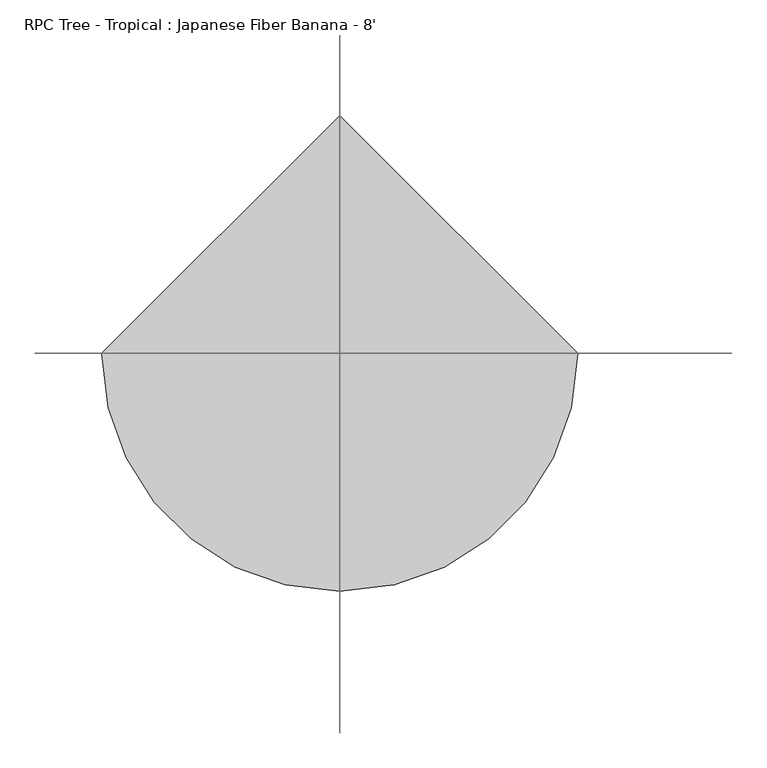
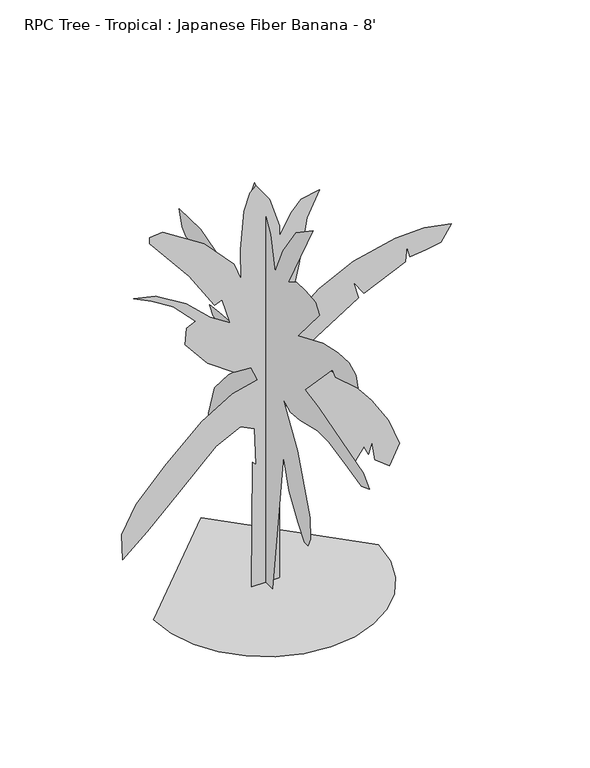
"""IFC4 building model written with IfcOpenShell, lengths in millimetres: geographic element geometry, RPC Tree - Tropical : Japanese Fiber Banana - 8'."""

from ifc_helpers import new_model, si_unit, origin, place, context, project, spatial, triangles, source, transform, mapped, element, save


def rpc_tree_tropical_japanese_fiber_banana_8_fc2fb2a9(model_context):
    return source(origin(), model_context, "Body", "Tessellation", [
        triangles([(-649.7467501, 0.0, 3.7e-06), (-632.5712723, -148.8792756, 3.7e-06), (-583.6506755, -285.6010629, 3.7e-06), (-506.9043426, -406.2488949, 3.7e-06), (-406.2488949, -506.9043426, 3.7e-06), (-285.6010629, -583.6506755, 3.7e-06), (-148.8792756, -632.5712723, 3.7e-06), (2.84e-05, -649.7467501, 3.7e-06), (148.8792756, -632.5712723, 3.7e-06), (285.6010629, -583.6506755, 3.7e-06), (406.2488949, -506.9043426, 3.7e-06), (506.9043426, -406.2488949, 3.7e-06), (583.6506755, -285.6010629, 3.7e-06), (632.5712723, -148.8790212, 3.7e-06), (649.7467501, 5.68e-05, 3.7e-06), (-8.52e-05, 649.7467501, 3.7e-06), (73.5169788, -2.4e-06, 1488.9400761), (86.1999983, -4e-06, 1501.9626823), (108.3956093, -6.3e-06, 1521.7797867), (138.5178168, -9.4e-06, 1547.2586094), (174.9816703, -1.3e-05, 1577.2688416), (216.2016834, -1.69e-05, 1610.6750874), (260.5921424, -2.12e-05, 1646.3444218), (306.5688237, -2.56e-05, 1683.149152), (505.0933339, -3.74e-05, 1782.4125698), (746.7776007, -4.41e-05, 1838.5162674), (915.0912369, -4.46e-05, 1842.831847), (1070.4584976, -4.1e-05, 1812.6209003), (1010.0392931, -3.02e-05, 1721.9908218), (923.7222507, -2.81e-05, 1704.7264687), (833.0921722, -2.71e-05, 1696.0954548), (815.8277464, -3.48e-05, 1760.832637), (807.1968052, -2.45e-05, 1674.5181381), (565.5150455, -1.17e-05, 1566.6237064), (505.0933339, -2.2e-05, 1652.9382053), (535.3041716, -9.6e-06, 1549.3592079), (250.4636001, 1.15e-05, 1372.4146305), (207.3058056, 2.02e-05, 1299.0465797), (457.6205775, 4.54e-05, 1087.573078), (608.672295, 6.81e-05, 897.679509), (707.9358582, 8.66e-05, 742.3123209), (772.6704969, 0.0001061, 578.3115755), (712.2512924, 0.00012, 461.7861663), (630.2496843, 0.0001123, 526.5233485), (612.9878019, 9.89e-05, 638.7333235), (591.4078691, 0.0001066, 573.9961049), (565.5150455, 0.0001, 630.1023823), (518.0422892, 0.0001082, 561.0496931), (237.5161527, 6.86e-05, 893.3640747), (99.411601, 4.9e-05, 1057.362204), (82.1486921, 4.08e-05, 1126.4148932), (77.8327038, 0.0001751, 0.0), (-81.8504909, 0.0001751, 0.0), (-77.5347659, 8.45e-05, 759.5742033), (-55.9558732, 8.71e-05, 737.996814), (-64.587582, 6.09e-05, 958.1012569), (-146.5871735, 5.57e-05, 1001.2585064), (-289.0071958, 6.39e-05, 932.2058172), (-500.4806794, 8.86e-05, 725.0478951), (-686.0587051, 0.0001097, 548.1032813), (-828.4769743, 0.0001241, 427.259858), (-832.7950247, 0.0001056, 582.6295896), (-750.7934166, 8.71e-05, 737.996814), (-573.8488029, 6.5e-05, 923.574876), (-371.0062786, 4.28e-05, 1109.1529381), (-194.0604295, 3e-05, 1217.044899), (-47.3244142, 2.59e-05, 1251.5712799), (-86.1662158, 1.56e-05, 1337.8882496), (-185.4289796, 1.46e-05, 1346.5192635), (-336.4799704, 1.7e-06, 1454.4136951), (-465.9543348, -1.73e-05, 1614.0963902), (-457.3233936, -2.87e-05, 1709.0419029), (-405.5326232, -3.18e-05, 1734.93727), (-535.0069877, -4.77e-05, 1868.7272141), (-660.1633381, -5.7e-05, 1946.4106991), (-763.7423355, -6.31e-05, 1998.1989624), (-638.583478, -5.95e-05, 1967.9881611), (-461.6388642, -4.67e-05, 1860.0962002), (-323.5335222, -3.12e-05, 1730.6218357), (-207.0078768, -2.25e-05, 1657.2536396), (-254.4808694, -4.1e-05, 1812.6209003), (-297.6381552, -3.9e-05, 1795.3590179), (-444.3744384, -6.62e-05, 2024.0943295), (-673.1097862, -9.91e-05, 2300.30247), (-673.1097862, -0.0001038, 2339.1442852), (-595.4261559, -0.0001043, 2343.4597195), (-358.0598668, -8.63e-05, 2192.4080383), (-185.4289796, -6.42e-05, 2006.8299763), (-142.2711851, -5.13e-05, 1898.9380154), (-146.5871735, -7.29e-05, 2080.198027), (-125.0082762, -0.0001002, 2308.9359547), (-90.4819498, -0.000112, 2408.1969017), (-55.9558732, -0.0001156, 2438.4078484), (21.7278389, -0.0001027, 2330.5132713), (77.8327038, -8.11e-05, 2149.2507889), (77.8327038, -7.39e-05, 2088.8315117), (146.8851113, -8.78e-05, 2205.3569572), (202.9900806, -9.5e-05, 2265.7760891), (310.8842943, -9.76e-05, 2287.3560219), (237.5161527, -8.01e-05, 2140.619775), (190.0426515, -4.87e-05, 1877.3580826), (142.5693864, -2.3e-05, 1661.5692192), (124.24932, -1.81e-05, 1620.2990639), (106.9864112, -1.34e-05, 1581.1042179), (91.8370452, -9.2e-06, 1546.0623161), (79.8586157, -5.8e-06, 1517.2485226), (72.1077807, -3.4e-06, 1496.740472), (69.6416885, -2.1e-06, 1486.6108578), (-6.07e-05, -228.3904198, 1972.5652073), (-6.46e-05, -305.2429235, 2016.4820034), (-6.49e-05, -396.7365758, 2020.139629), (-6.39e-05, -495.5454429, 2009.1616653), (-5.9e-05, -535.8019973, 1954.2670509), (-3.61e-05, -319.883527, 1698.0893738), (-4.56e-05, -568.7408298, 1804.2211224), (-4.86e-05, -718.786722, 1837.1573387), (-4.89e-05, -828.5760235, 1840.8175804), (-4.63e-05, -901.771483, 1811.5388443), (-4.01e-05, -920.0697121, 1742.0061699), (-3.38e-05, -696.8283966, 1672.4708794), (-3.65e-05, -667.5522039, 1701.7496155), (-1.06e-05, -393.0764068, 1412.635722), (-8.3e-06, -524.8241063, 1387.0172276), (3.5e-06, -974.9643265, 1255.2694553), (8.7e-06, -1037.1792789, 1196.7146719), (1.13e-05, -956.6660975, 1167.4360085), (8.7e-06, -821.2583015, 1196.7146719), (5.1e-06, -623.6354805, 1236.971299), (5.1e-06, -517.5038046, 1236.971299), (8.7e-06, -341.8393816, 1196.7146719), (9.7e-06, -246.688885, 1185.7342375), (6.4e-06, -169.8356182, 1222.3306229), (2.67e-05, -316.2233943, 995.4317545), (5.65e-05, -440.6507558, 662.4010649), (6.79e-05, -447.9710575, 534.3135707), (7.28e-05, -422.3525631, 479.4163765), (7.28e-05, -385.756105, 479.4163765), (6.53e-05, -323.5411526, 563.5896907), (5.32e-05, -232.0500619, 698.9975229), (3.75e-05, -177.1549025, 874.6619459), (5.84e-05, -147.8774926, 640.4427395), (0.0001157, -67.36457, 3.7e-06), (0.0001157, 82.6820898, 3.7e-06), (9.61e-05, 82.6820898, 219.5804016), (0.0001026, 64.3836201, 146.3870222), (7.84e-05, 35.1062147, 417.2039675), (4.99e-05, 35.1062147, 735.593981), (2.38e-05, 79.0221933, 1028.3680435), (2.8e-05, 174.1739435, 980.7936945), (4.14e-05, 331.5396469, 830.7452225), (5.19e-05, 430.3510211, 713.6355829), (5.84e-05, 444.9891174, 640.4427395), (5.58e-05, 470.6076118, 669.7214029), (6.33e-05, 466.9474792, 585.5480887), (6.01e-05, 529.1624316, 622.1445105), (6.5e-05, 551.1207933, 567.2498597), (5.45e-05, 573.0791914, 684.3594629), (3.75e-05, 514.5243716, 874.6619459), (2.28e-05, 375.4563704, 1039.3484779), (6.1e-06, 170.5143013, 1225.9908646), (1.8e-06, 272.9848271, 1273.567757), (-1.1e-06, 393.7545994, 1306.5039734), (2e-07, 459.6297209, 1291.8659134), (-1.1e-06, 529.1624316, 1306.5039734), (-5e-06, 565.7588533, 1350.4207695), (-6.4e-06, 466.9474792, 1365.0588295), (-7.7e-06, 254.6866163, 1379.6968895), (-1.32e-05, 331.5396469, 1441.911842), (-2.5e-05, 514.5243716, 1573.6594688), (-2.96e-05, 730.4453854, 1624.896603), (-2.96e-05, 799.9781324, 1624.896603), (-3.29e-05, 840.2346869, 1661.4929157), (-4.1e-05, 869.5133503, 1752.9841335), (-4.14e-05, 653.5923729, 1756.6442299), (-3.58e-05, 441.3289484, 1694.4292774), (-3.02e-05, 283.9652797, 1632.214325), (-1.62e-05, 108.2998484, 1474.8480583), (-5.35e-05, 152.215827, 1892.0520985), (-8.06e-05, 185.15287, 2195.804052), (-9.63e-05, 111.9594906, 2371.468475), (-9.01e-05, 46.0854001, 2301.9356552), (-7.67e-05, -45.4067079, 2151.889872), (-5.87e-05, -89.322691, 1950.6068092), (-7.44e-05, -169.8356182, 2126.2712322), (-9.14e-05, -301.5827909, 2316.5737152), (-0.0001016, -469.9294556, 2430.0231857)], [[15, 16, 1], [14, 15, 1], [14, 1, 2], [13, 14, 2], [13, 2, 3], [13, 3, 4], [12, 13, 4], [11, 12, 4], [11, 4, 5], [11, 5, 6], [11, 6, 7], [11, 7, 8], [11, 8, 9], [11, 9, 10], [75, 76, 77], [45, 46, 47], [53, 54, 55], [60, 61, 62], [98, 99, 100], [97, 98, 100], [27, 28, 29], [27, 29, 30], [47, 48, 49], [60, 62, 63], [59, 60, 63], [59, 63, 64], [58, 59, 64], [58, 64, 65], [74, 75, 77], [74, 77, 78], [73, 74, 78], [73, 78, 79], [42, 43, 44], [42, 44, 45], [41, 42, 45], [92, 93, 94], [91, 92, 94], [96, 97, 100], [96, 100, 101], [52, 53, 55], [51, 52, 55], [51, 55, 56], [57, 58, 65], [57, 65, 66], [57, 66, 67], [27, 30, 31], [27, 31, 32], [26, 27, 32], [84, 85, 86], [83, 84, 86], [83, 86, 87], [83, 87, 88], [82, 83, 88], [81, 82, 88], [81, 88, 89], [56, 57, 67], [51, 56, 67], [91, 94, 95], [90, 91, 95], [90, 95, 96], [89, 90, 96], [89, 96, 101], [89, 101, 102], [33, 34, 35], [32, 33, 35], [26, 32, 35], [25, 26, 35], [24, 25, 35], [81, 89, 102], [80, 81, 102], [80, 102, 103], [80, 103, 104], [80, 104, 105], [80, 105, 106], [80, 106, 107], [40, 41, 45], [40, 45, 47], [40, 47, 49], [39, 40, 49], [38, 39, 49], [38, 49, 50], [38, 50, 51], [38, 51, 67], [38, 67, 68], [35, 36, 37], [24, 35, 37], [23, 24, 37], [22, 23, 37], [21, 22, 37], [20, 21, 37], [19, 20, 37], [18, 19, 37], [17, 18, 37], [17, 37, 38], [17, 38, 68], [108, 17, 68], [80, 107, 108], [80, 108, 68], [80, 68, 69], [80, 69, 70], [80, 70, 71], [79, 80, 71], [73, 79, 71], [73, 71, 72], [143, 144, 145], [185, 186, 109], [184, 185, 109], [155, 156, 157], [183, 184, 109], [151, 152, 153], [153, 154, 155], [164, 165, 166], [163, 164, 166], [124, 125, 126], [179, 180, 181], [172, 173, 174], [171, 172, 174], [170, 171, 174], [169, 170, 174], [169, 174, 175], [142, 143, 145], [141, 142, 145], [141, 145, 146], [141, 146, 147], [140, 141, 147], [140, 147, 148], [162, 163, 166], [162, 166, 167], [161, 162, 167], [179, 181, 182], [178, 179, 182], [178, 182, 183], [153, 155, 157], [153, 157, 158], [151, 153, 158], [150, 151, 158], [150, 158, 159], [149, 150, 159], [149, 159, 160], [148, 149, 160], [124, 126, 127], [123, 124, 127], [123, 127, 128], [123, 128, 129], [118, 119, 120], [117, 118, 120], [116, 117, 120], [116, 120, 121], [115, 116, 121], [115, 121, 122], [114, 115, 122], [168, 169, 175], [168, 175, 176], [168, 176, 177], [167, 168, 177], [177, 178, 183], [122, 123, 129], [122, 129, 130], [112, 113, 114], [111, 112, 114], [110, 111, 114], [109, 110, 114], [183, 109, 114], [177, 183, 114], [177, 114, 122], [177, 122, 130], [177, 130, 131], [177, 131, 132], [167, 177, 132], [161, 167, 132], [160, 161, 132], [148, 160, 132], [140, 148, 132], [140, 132, 133], [140, 133, 134], [139, 140, 134], [138, 139, 134], [138, 134, 135], [137, 138, 135], [137, 135, 136]], closed=False),
    ])


if __name__ == "__main__":
    model = new_model("IFC4")
    model_context = context("Model", 3, world=origin())
    ifc_project = project(units=[si_unit("LENGTHUNIT", "METRE", prefix="MILLI")], contexts=[model_context])
    site = spatial("IfcSite", under=ifc_project)
    building = spatial("IfcBuilding", under=site)
    placement = place(None, origin())
    rpc_tree_tropical_japanese_fiber_banana_8_shape = rpc_tree_tropical_japanese_fiber_banana_8_fc2fb2a9(model_context)
    element("IfcGeographicElement", 1, ObjectType="RPC Tree - Tropical : Japanese Fiber Banana - 8'", at=placement, inside=building, context=model_context, shape_type="MappedRepresentation", body=[
        mapped(rpc_tree_tropical_japanese_fiber_banana_8_shape, transform((0.0, 0.0, 0.0), x_axis=(1.0, 0.0, 0.0), y_axis=(0.0, 1.0, 0.0), z_axis=(0.0, 0.0, 1.0))),
    ])
    save(model, "model.ifc")

# Revit data of these elements
# Type "RPC Tree - Tropical : Japanese Fiber Banana - 8'"
#   built-in parameter 1005198 = "{2, 15},{39, RPC-16-FVGT-NR7X-7G1M-A000-ST1L-LVER-AU},{1, 0},{1, 0},{2, 35},{1, 8},{5, Color},{1, 0},{1, 0},{3, 0.8},{3, 0.8},{3, 0.8},{1, 8},{7, BBoxMin},{1, 0},{1, 0},{1, 0},{1, 0},{1, 0},{1, 8},{7, BBoxMax},{1, 0},{1, 0},{1, 0},{1, 0},{1, 0},{2, 11},{9, RPCTypeId},{1, 0},{1, 0},{39, RPC-16-FVGT-NR7X-7G1M-A000-ST1L-LVER-AU},{1, 6},{14, RPCPlantHeight},{1, 0},{1, 0},{1, 8},{2, 11},{7, keyword},{1, 0},{1, 0},{62, :Geometry:RPC:Japanese Fiber Banana:Musa basjoo:Tree:Tropical.},{2, 11},{8, category},{1, 0},{1, 0},{17, :Trees [Tropical]},{2, 11},{12, LocalizedUID},{1, 0},{1, 0},{21, Japanese Fiber Banana},{2, 14},{6, Height},{1, 0},{1, 0},{1, 8},{1, 2},{16, Cast Reflections},{1, 0},{1, 0},{1, 0},{1, 2},{12, Cast Shadows},{1, 0},{1, 0},{1, 1},{1, 2},{9, Lock View},{1, 0},{1, 0},{1, 0},{1, 4},{5, ViewC},{1, 0},{1, 0},{1, 0},{2, 11},{20, AdvancedUIDefinition},{1, 0},{1, 0},{0, },{2, 11},{10, AssetLibID},{1, 0},{1, 0},{36, 4D3F6E72-3F99-4203-98E9-AF80B3C7A7A4},{2, 11},{10, BaseSchema},{1, 0},{1, 0},{9, RPCSchema},{2, 11},{12, ExchangeGUID},{1, 0},{1, 0},{0, },{1, 2},{6, Hidden},{1, 0},{1, 0},{1, 0},{1, 4},{11, RPCCategory},{1, 0},{1, 0},{1, 0},{2, 11},{8, RPCImage},{1, 0},{1, 0},{0, },{1, 4},{13, SchemaVersion},{1, 0},{1, 0},{1, 4},{2, 11},{12, UIDefinition},{1, 0},{1, 0},{0, },{2, 11},{6, UIName},{1, 0},{1, 0},{39, RPC-16-FVGT-NR7X-7G1M-A000-ST1L-LVER-AU},{2, 11},{11, VersionGUID},{1, 0},{1, 0},{9, RPCSchema},{2, 11},{9, assettype},{1, 0},{1, 0},{11, RPCGeometry},{2, 11},{11, description},{1, 0},{1, 0},{0, },{2, 11},{9, localname},{1, 0},{1, 0},{3, RPC},{2, 11},{9, localtype},{1, 0},{1, 0},{3, RPC},{1, 4},{8, revision},{1, 0},{1, 0},{1, 1},{2, 11},{9, thumbnail},{1, 0},{1, 0},{0, },{1, 4},{7, version},{1, 0},{1, 0},{1, 1},{1, 2},{20, RPC_Cast Reflections},{1, 0},{1, 0},{1, 1},{1, 2},{16, RPC_Cast Shadows},{1, 0},{1, 0},{1, 1},{1, 2},{13, RPC_Lock View},{1, 0},{1, 0},{1, 0},{1, 4},{9, RPC_ViewC},{1, 0},{1, 0},{1, 0},{21, assetlibrary_base.fbx},{1, 5},"
#   built-in parameter 1005195 = "RPC-16-FVGT-NR7X-7G1M-A000-ST1L-LVER-AU"
#   Type Comments = "Japanese Fiber Banana"
#   Assembly Code = "G2050500"
#   Height = 8' - 0"
#   Plan Symbol = element 455244
#   Default Elevation = 0
